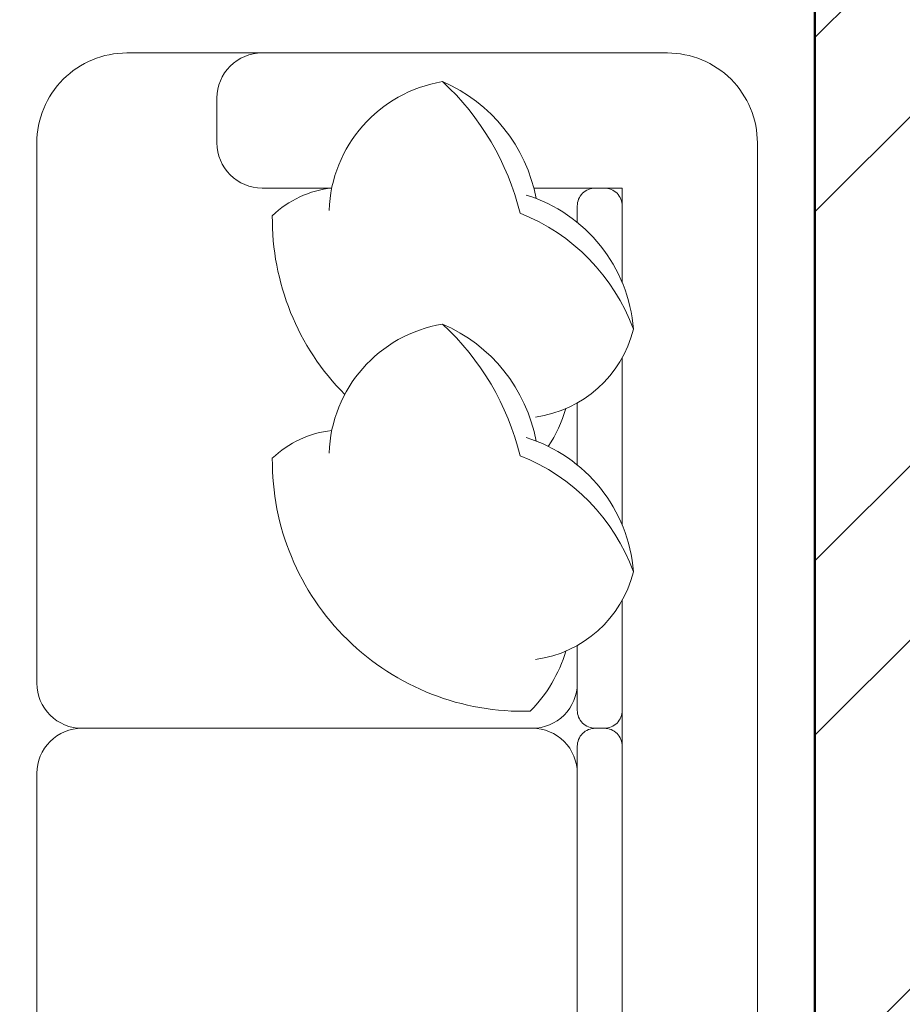
# Model space of a CAD drawing. Units: inches. Extents: x 963 to 2075, y 289 to 2657.
# Tile 76 of 98: x 1488 to 1511, y 2265 to 2290. Entities that reach past the tile are written whole.
import ezdxf

# ---------------------------------------------------------------- set-up
doc = ezdxf.new("R2010")
doc.units = ezdxf.units.IN
for name, color, linetype, lineweight in [('A-FURN', 8, 'Continuous', 18), ('A-WALL', 7, 'Continuous', 50), ('A-WALL-PATT', 8, 'Continuous', 13)]:
    doc.layers.add(name, color=color, linetype=linetype, lineweight=lineweight)

msp = doc.modelspace()

# ---------------------------------------------------------------- hatches: boundary and pattern name
at = {"layer": 'A-WALL-PATT'}
h = msp.add_hatch(dxfattribs=at)
h.set_pattern_fill('ANSI32', color=256)
h.paths.add_polyline_path([(1296.922, 2558.318), (1203.922, 2558.318), (1203.922, 2493.818), (1191.533, 2493.818), (1191.533, 2489.318), (1211.063, 2489.318), (1211.063, 2492.02), (1211.063, 2493.818), (1208.422, 2493.818), (1208.422, 2553.818), (1292.422, 2553.818), (1292.422, 2538.863), (1296.922, 2538.863)])
h.paths.add_polyline_path([(1442.422, 2558.318), (1349.422, 2558.318), (1349.422, 2538.943), (1353.922, 2538.943), (1353.922, 2553.818), (1437.922, 2553.818), (1437.922, 2493.818), (1434.542, 2493.818), (1434.542, 2489.318), (1448.311, 2489.318), (1448.311, 2491.568), (1448.311, 2493.818), (1442.422, 2493.818)])
h.paths.add_polyline_path([(1415.554, 2491.568), (1415.554, 2493.818), (1340.941, 2493.818), (1340.941, 2489.318), (1371.922, 2489.318), (1371.922, 2378.318), (1367.596, 2378.318), (1367.596, 2373.818), (1371.922, 2373.818), (1371.922, 2355.185), (1376.422, 2355.185), (1376.422, 2489.318), (1415.554, 2489.318)])
h.paths.add_polyline_path([(1304.941, 2491.568), (1304.941, 2493.818), (1296.922, 2493.818), (1296.922, 2514.863), (1292.422, 2514.863), (1292.422, 2493.818), (1232.808, 2493.818), (1232.808, 2489.318), (1256.422, 2489.318), (1256.422, 2327.318), (1253.714, 2327.318), (1253.714, 2322.818), (1328.422, 2322.818), (1328.422, 2331.147), (1323.922, 2331.147), (1323.922, 2327.318), (1260.922, 2327.318), (1260.922, 2373.818), (1323.922, 2373.818), (1323.922, 2357.812), (1328.422, 2357.812), (1328.422, 2373.818), (1346.007, 2373.818), (1346.007, 2376.068), (1346.007, 2378.318), (1260.922, 2378.318), (1260.922, 2489.318), (1304.941, 2489.318)])
h.paths.add_polyline_path([(1226.654, 2327.318), (1124.422, 2327.318), (1124.422, 2347.447), (1119.922, 2347.447), (1119.922, 2322.818), (1163.422, 2322.818), (1163.422, 2305.435), (1165.672, 2305.435), (1167.922, 2305.435), (1167.922, 2322.818), (1226.654, 2322.818), (1226.654, 2325.068)])
h.paths.add_polyline_path([(1095.922, 2489.318), (1124.422, 2489.318), (1131.533, 2489.318), (1131.533, 2491.568), (1131.533, 2493.818), (1119.922, 2493.818), (1091.422, 2493.818), (1091.422, 2417.318), (1095.922, 2417.318), (1119.922, 2417.318), (1119.922, 2407.447), (1124.422, 2407.447), (1124.422, 2421.818), (1095.922, 2421.818)])
h.paths.add_polyline_path([(1512.922, 2558.318), (1508.422, 2558.318), (1508.422, 2493.818), (1503.401, 2493.818), (1503.401, 2489.318), (1508.422, 2489.318), (1508.422, 2327.318), (1376.422, 2327.318), (1376.422, 2330.273), (1371.922, 2330.273), (1371.922, 2298.744), (1376.422, 2298.744), (1376.422, 2322.818), (1508.422, 2322.818), (1508.422, 2165.318), (1504.255, 2165.318), (1504.255, 2160.818), (1508.422, 2160.818), (1508.422, 2108.318), (1512.922, 2108.318), (1512.922, 2160.818), (1516.182, 2160.818), (1516.182, 2163.068), (1516.182, 2165.318), (1512.922, 2165.318), (1512.922, 2322.818), (1644.922, 2322.818), (1644.922, 2298.744), (1649.422, 2298.744), (1649.422, 2322.818), (1649.422, 2330.944), (1647.172, 2330.944), (1644.922, 2330.944), (1644.922, 2327.318), (1512.922, 2327.318), (1512.922, 2489.318), (1516.759, 2489.318), (1516.759, 2491.568), (1516.759, 2493.818), (1512.922, 2493.818)])
h.paths.add_polyline_path([(1671.922, 2558.318), (1578.922, 2558.318), (1578.922, 2493.818), (1573.526, 2493.818), (1573.526, 2489.318), (1586.537, 2489.318), (1586.537, 2491.568), (1586.537, 2493.818), (1583.422, 2493.818), (1583.422, 2553.818), (1667.422, 2553.818), (1667.422, 2541.109), (1671.922, 2541.109)])
h.paths.add_polyline_path([(1681.257, 2493.818), (1671.922, 2493.818), (1671.922, 2517.109), (1667.422, 2517.109), (1667.422, 2493.818), (1610.218, 2493.818), (1610.218, 2489.318), (1644.922, 2489.318), (1644.922, 2357.865), (1649.422, 2357.865), (1649.422, 2373.818), (1652.203, 2373.818), (1652.203, 2375.827), (1652.203, 2378.318), (1649.422, 2378.318), (1649.422, 2489.318), (1681.257, 2489.318), (1681.257, 2491.568)])
h.paths.add_polyline_path([(1821.922, 2558.318), (1728.922, 2558.318), (1728.922, 2541), (1733.422, 2541), (1733.422, 2553.818), (1817.422, 2553.818), (1817.422, 2493.818), (1813.507, 2493.818), (1813.507, 2489.318), (1830.078, 2489.318), (1830.078, 2491.568), (1830.078, 2493.818), (1821.922, 2493.818)])
h.paths.add_polyline_path([(1794.244, 2493.818), (1717.257, 2493.818), (1717.257, 2489.318), (1760.422, 2489.318), (1760.422, 2378.318), (1674.401, 2378.318), (1674.401, 2373.818), (1692.922, 2373.818), (1692.922, 2356.954), (1697.422, 2356.954), (1697.422, 2373.818), (1760.422, 2373.818), (1760.422, 2327.318), (1697.422, 2327.318), (1697.422, 2333.341), (1692.922, 2333.341), (1692.922, 2322.818), (1768.037, 2322.818), (1768.037, 2325.068), (1768.037, 2327.318), (1764.922, 2327.318), (1764.922, 2489.318), (1794.244, 2489.318)])
h.paths.add_polyline_path([(1733.422, 2517), (1728.922, 2517), (1728.922, 2493.818), (1733.422, 2493.818)], flags=17)
h.paths.add_polyline_path([(1929.922, 2493.818), (1890.078, 2493.818), (1890.078, 2489.318), (1896.922, 2489.318), (1925.422, 2489.318), (1925.422, 2421.818), (1896.922, 2421.818), (1896.922, 2408.318), (1901.422, 2408.318), (1901.422, 2417.318), (1925.422, 2417.318), (1929.922, 2417.318)])
h.paths.add_polyline_path([(1901.422, 2348.318), (1896.922, 2348.318), (1896.922, 2327.318), (1800.423, 2327.318), (1800.423, 2322.818), (1853.422, 2322.818), (1853.422, 2309.453), (1857.922, 2309.453), (1857.922, 2322.818), (1901.422, 2322.818)])
h.paths.add_polyline_path([(1857.922, 2249.453), (1853.422, 2249.453), (1853.422, 2214.818), (1686.309, 2214.818), (1686.309, 2210.318), (1853.422, 2210.318), (1853.422, 2202.134), (1857.922, 2202.134), (1857.922, 2210.318)])
h.paths.add_polyline_path([(1857.922, 2142.134), (1853.422, 2142.134), (1853.422, 2115.422), (1841.422, 2115.422), (1841.422, 2088.531), (1841.422, 2046.949), (1845.922, 2046.949), (1845.922, 2110.922), (1905.922, 2110.922), (1905.922, 2092.517), (1910.422, 2092.517), (1910.422, 2115.422), (1857.922, 2115.422)])
h.paths.add_polyline_path([(1532.436, 1482.342), (1573.456, 1482.342), (1573.456, 1501), (1532.436, 1501)], flags=9)
h.paths.add_polyline_path([(1438.658, 1486.302), (1479.678, 1486.302), (1479.678, 1504.96), (1438.658, 1504.96)], flags=9)
h.paths.add_polyline_path([(1411.215, 1365.308), (1659.139, 1365.308), (1659.139, 1402.401), (1411.215, 1402.401)], flags=9)
h.paths.add_polyline_path([(1185.671, 2296.298), (1248.16, 2296.298), (1248.16, 2314.955), (1185.671, 2314.955)], flags=9)
h.paths.add_polyline_path([(1177.31, 2187.35), (1216.15, 2187.35), (1216.15, 2206.007), (1177.31, 2206.007)], flags=9)
h.paths.add_polyline_path([(1295.101, 1602.083), (1328.26, 1602.083), (1328.26, 1620.741), (1295.101, 1620.741)], flags=9)
h.paths.add_polyline_path([(1525.126, 2005.99), (1558.39, 2005.99), (1558.39, 2024.648), (1525.126, 2024.648)], flags=9)
h.paths.add_polyline_path([(1459.606, 1977.125), (1472.195, 1977.125), (1472.195, 1987.429), (1459.606, 1987.429)], flags=9)
h.paths.add_polyline_path([(1467.815, 2053.676), (1480.018, 2053.676), (1480.018, 2063.979), (1467.815, 2063.979)], flags=9)
h.paths.add_polyline_path([(1555.184, 2119.02), (1584.563, 2119.02), (1584.563, 2137.678), (1555.184, 2137.678)], flags=25)
h.paths.add_polyline_path([(1405.389, 2115.291), (1444.478, 2115.291), (1444.478, 2133.948), (1405.389, 2133.948)], flags=25)
h.paths.add_polyline_path([(1698.482, 2004.259), (1727.695, 2004.259), (1727.695, 2022.916), (1698.482, 2022.916)], flags=9)
h.paths.add_polyline_path([(1612.158, 1972.855), (1629.016, 1972.855), (1629.016, 1983.159), (1612.158, 1983.159)], flags=9)
h.paths.add_polyline_path([(1608.289, 2060.036), (1625.147, 2060.036), (1625.147, 2070.34), (1608.289, 2070.34)], flags=9)
h.paths.add_polyline_path([(1527.954, 1684.402), (1566.795, 1684.402), (1566.795, 1703.06), (1527.954, 1703.06)], flags=9)
h.paths.add_polyline_path([(1422.792, 1683.59), (1461.633, 1683.59), (1461.633, 1702.247), (1422.792, 1702.247)], flags=9)
h.paths.add_polyline_path([(1531.262, 1732.459), (1574.015, 1732.459), (1574.015, 1751.116), (1531.262, 1751.116)], flags=9)
h.paths.add_polyline_path([(1402.872, 1732.845), (1439.799, 1732.845), (1439.799, 1751.502), (1402.872, 1751.502)], flags=9)
h.paths.add_polyline_path([(1243.122, 1923.132), (1281.962, 1923.132), (1281.962, 1941.79), (1243.122, 1941.79)], flags=9)
h.paths.add_polyline_path([(1181.752, 1792.268), (1244.241, 1792.268), (1244.241, 1810.926), (1181.752, 1810.926)], flags=9)
h.paths.add_polyline_path([(1265.822, 1670.3), (1316.071, 1670.3), (1316.071, 1688.957), (1265.822, 1688.957)], flags=9)
h.paths.add_polyline_path([(1140.263, 1676.054), (1179.104, 1676.054), (1179.104, 1694.711), (1140.263, 1694.711)], flags=9)
h.paths.add_polyline_path([(1107.49, 1490.889), (1143.374, 1490.889), (1143.374, 1509.546), (1107.49, 1509.546)], flags=9)
h.paths.add_polyline_path([(1217.584, 1483.899), (1246.741, 1483.899), (1246.741, 1502.556), (1217.584, 1502.556)], flags=9)
h.paths.add_polyline_path([(1389.21, 1486.919), (1418.367, 1486.919), (1418.367, 1505.576), (1389.21, 1505.576)], flags=9)
h.paths.add_polyline_path([(1672.208, 1602.083), (1705.366, 1602.083), (1705.366, 1620.741), (1672.208, 1620.741)], flags=9)
h.paths.add_polyline_path([(1752.082, 1522.638), (1781.24, 1522.638), (1781.24, 1541.295), (1752.082, 1541.295)], flags=9)
h.paths.add_polyline_path([(1848.275, 1491.26), (1884.158, 1491.26), (1884.158, 1509.918), (1848.275, 1509.918)], flags=9)
h.paths.add_polyline_path([(1822.47, 1685.62), (1861.31, 1685.62), (1861.31, 1704.278), (1822.47, 1704.278)], flags=9)
h.paths.add_polyline_path([(1713.195, 1672.232), (1763.444, 1672.232), (1763.444, 1690.889), (1713.195, 1690.889)], flags=9)
h.paths.add_polyline_path([(1736.619, 1790.578), (1799.109, 1790.578), (1799.109, 1809.235), (1736.619, 1809.235)], flags=9)
h.paths.add_polyline_path([(1691.491, 1916.355), (1730.332, 1916.355), (1730.332, 1935.013), (1691.491, 1935.013)], flags=9)
h.paths.add_polyline_path([(1764.872, 1973.922), (1794.306, 1973.922), (1794.306, 1992.58), (1764.872, 1992.58)], flags=9)
h.paths.add_polyline_path([(1767.854, 2034.017), (1797.288, 2034.017), (1797.288, 2052.674), (1767.854, 2052.674)], flags=9)
h.paths.add_polyline_path([(1851.593, 2060.331), (1880.751, 2060.331), (1880.751, 2078.989), (1851.593, 2078.989)], flags=25)
h.paths.add_polyline_path([(1688.491, 2086.874), (1727.332, 2086.874), (1727.332, 2105.531), (1688.491, 2105.531)], flags=9)
h.paths.add_polyline_path([(1537.743, 2293.581), (1580.495, 2293.581), (1580.495, 2312.239), (1537.743, 2312.239)], flags=25)
h.paths.add_polyline_path([(1425.587, 2296.109), (1468.34, 2296.109), (1468.34, 2314.766), (1425.587, 2314.766)], flags=25)
h.paths.add_polyline_path([(1278.518, 2004.184), (1307.72, 2004.184), (1307.72, 2022.841), (1278.518, 2022.841)], flags=9)
h.paths.add_polyline_path([(1193.282, 1973.635), (1222.715, 1973.635), (1222.715, 1992.292), (1193.282, 1992.292)], flags=9)
h.paths.add_polyline_path([(1192.411, 2040.577), (1221.845, 2040.577), (1221.845, 2059.234), (1192.411, 2059.234)], flags=9)
h.paths.add_polyline_path([(1130.603, 1951.393), (1159.76, 1951.393), (1159.76, 1970.05), (1130.603, 1970.05)], flags=9)
h.paths.add_polyline_path([(1132.827, 2052.494), (1161.984, 2052.494), (1161.984, 2071.151), (1132.827, 2071.151)], flags=9)
h.paths.add_polyline_path([(1265.128, 2334.619), (1315.377, 2334.619), (1315.377, 2353.277), (1265.128, 2353.277)], flags=25)
h.paths.add_polyline_path([(1136.741, 2330.785), (1175.582, 2330.785), (1175.582, 2349.443), (1136.741, 2349.443)], flags=9)
h.paths.add_polyline_path([(1287.422, 2417.204), (1320.58, 2417.204), (1320.58, 2435.861), (1287.422, 2435.861)], flags=25)
h.paths.add_polyline_path([(1430.988, 2329.159), (1469.828, 2329.159), (1469.828, 2347.816), (1430.988, 2347.816)], flags=25)
h.paths.add_polyline_path([(1525.424, 2329.213), (1564.264, 2329.213), (1564.264, 2347.87), (1525.424, 2347.87)], flags=25)
h.paths.add_polyline_path([(1684.525, 2382.799), (1717.683, 2382.799), (1717.683, 2401.457), (1684.525, 2401.457)], flags=25)
h.paths.add_polyline_path([(1704.805, 2340.293), (1755.054, 2340.293), (1755.054, 2358.95), (1704.805, 2358.95)], flags=25)
h.paths.add_polyline_path([(1694.113, 2287.757), (1756.602, 2287.757), (1756.602, 2306.414), (1694.113, 2306.414)], flags=9)
h.paths.add_polyline_path([(1815.778, 2329.861), (1854.618, 2329.861), (1854.618, 2348.518), (1815.778, 2348.518)], flags=9)
h.paths.add_polyline_path([(1842.873, 2514.256), (1878.756, 2514.256), (1878.756, 2532.914), (1842.873, 2532.914)], flags=9)
h.paths.add_polyline_path([(1769.513, 2531.447), (1798.671, 2531.447), (1798.671, 2550.104), (1769.513, 2550.104)], flags=25)
h.paths.add_polyline_path([(1594.772, 2518.468), (1623.93, 2518.468), (1623.93, 2537.125), (1594.772, 2537.125)], flags=25)
h.paths.add_polyline_path([(1520.723, 2516.185), (1556.606, 2516.185), (1556.606, 2534.842), (1520.723, 2534.842)], flags=25)
h.paths.add_polyline_path([(1464.456, 2516.694), (1500.34, 2516.694), (1500.34, 2535.351), (1464.456, 2535.351)], flags=25)
h.paths.add_polyline_path([(1365.696, 2528.97), (1394.854, 2528.97), (1394.854, 2547.627), (1365.696, 2547.627)], flags=25)
h.paths.add_polyline_path([(1222.838, 2516.231), (1251.995, 2516.231), (1251.995, 2534.889), (1222.838, 2534.889)], flags=25)
h.paths.add_polyline_path([(1104.545, 2509.6), (1140.429, 2509.6), (1140.429, 2528.257), (1104.545, 2528.257)], flags=9)

# ---------------------------------------------------------------- linework, layer by layer
at = {"layer": 'A-FURN', "ltscale": 0.03}
msp.add_lwpolyline([(1490.72, 2240.636, -0.414214), (1488.403, 2242.954), (1488.403, 2256.859, -0.414214), (1489.562, 2258.018, -0.414214), (1488.403, 2259.177), (1488.403, 2270.765, -0.414214), (1489.562, 2271.924, -0.414214), (1488.403, 2273.082), (1488.403, 2286.988, -0.414214), (1490.72, 2289.306), (1504.626, 2289.306, -0.414214), (1506.944, 2286.988), (1506.944, 2242.954, -0.414214), (1504.626, 2240.636)], format="xyb", close=True, dxfattribs=at)
at = {"layer": 'A-FURN'}
for points in [[(1495.992, 2285.829), (1494.197, 2285.829, -0.414214), (1493.038, 2286.988), (1493.038, 2288.147, -0.414214), (1494.197, 2289.306)], [(1495.922, 2285.248, -0.356772), (1498.843, 2288.568, -0.249542), (1501.25, 2285.56, 9.61688)], [(1498.843, 2288.568, -0.14773), (1500.835, 2285.181, -0.213343), (1503.755, 2282.193, -0.178662)], [(1495.993, 2285.832, 0.165541), (1494.462, 2285.115, 0.200231), (1496.326, 2280.515, 0.121523)], [(1500.993, 2285.649, -0.306663), (1503.755, 2282.193, -0.30633), (1501.233, 2279.935, 0.872847)], [(1503.467, 2283.392), (1503.467, 2285.829), (1501.19, 2285.829, -0.414214)], [(1502.308, 2284.945), (1502.308, 2285.366, -0.414214), (1502.772, 2285.829), (1503.004, 2285.829, -0.414214), (1503.467, 2285.366)], [(1503.467, 2285.366), (1503.467, 2283.392, -0.414214)], [(1495.922, 2279.005, -0.356772), (1498.843, 2282.326, -0.249542), (1501.25, 2279.317, 9.61688)], [(1498.843, 2282.326, -0.14773), (1500.835, 2278.939, -0.213343), (1503.755, 2275.951, -0.178662)], [(1503.467, 2281.464), (1503.467, 2277.149, -0.414214)], [(1501.562, 2279.18, 0.071865), (1502.015, 2280.152, -7.115464)], [(1502.308, 2278.703), (1502.308, 2280.297, -0.414214)], [(1495.993, 2279.589, 0.165541), (1494.462, 2278.873, 0.425989), (1501.1, 2272.364, 0.121523), (1502.015, 2273.909, -7.115464)], [(1500.993, 2279.407, -0.306663), (1503.755, 2275.951, -0.30633), (1501.233, 2273.693, 0.872847)], [(1503.467, 2275.221), (1503.467, 2272.387, -0.414214), (1503.004, 2271.924), (1502.772, 2271.924, -0.414214), (1502.308, 2272.387), (1502.308, 2274.054, -0.414214)], [(1502.308, 2273.082, -0.414214), (1501.15, 2271.924), (1489.562, 2271.924, -0.414214)], [(1502.308, 2270.765, 0.414214), (1501.15, 2271.924)]]:
    msp.add_lwpolyline(points, format="xyb", dxfattribs=at)
for points in [[(1503.467, 2277.149), (1503.467, 2281.464)], [(1503.467, 2248.478), (1503.467, 2275.221)]]:
    msp.add_lwpolyline(points, dxfattribs=at)
msp.add_lwpolyline([(1503.467, 2271.46), (1503.467, 2258.482, -0.414214), (1503.004, 2258.018), (1502.772, 2258.018, -0.414214), (1502.308, 2258.482), (1502.308, 2271.46, -0.414214), (1502.772, 2271.924), (1503.004, 2271.924, -0.414214)], format="xyb", close=True, dxfattribs=at)
at = {"layer": 'A-WALL'}
msp.add_line((1508.422, 2322.818), (1508.422, 2165.318), dxfattribs=at)

doc.saveas('drawing.dxf')
